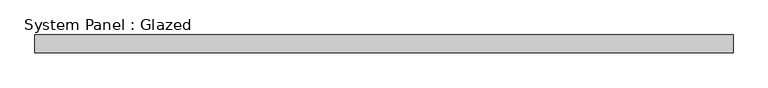
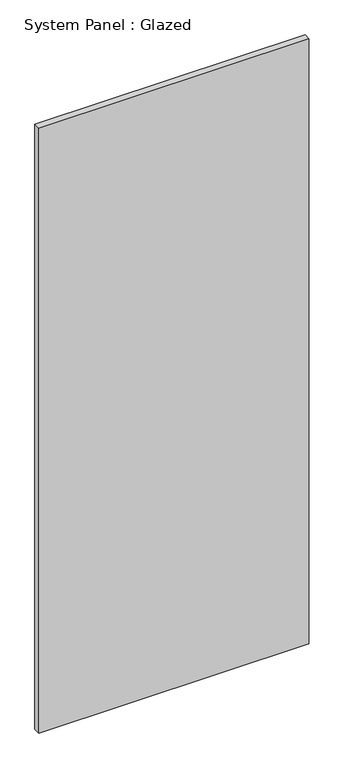
"""IFC4 building model written with IfcOpenShell, lengths in millimetres: plate geometry, System Panel : Glazed."""

from ifc_helpers import new_model, si_unit, origin, origin_with_axes, place, context, project, spatial, polyline, outline, extrude, source, transform, mapped, element, save


def system_panel_glazed_9df4f396(model_context):
    return source(origin(), model_context, "Body", "SweptSolid", [
        extrude(outline(polyline([(501.65, 19.05), (-501.65, 19.05), (-501.65, 44.45), (501.65, 44.45), (501.65, 19.05)])), origin_with_axes(), (0.0, 0.0, 1.0), 2374.9),
    ])


if __name__ == "__main__":
    model = new_model("IFC4")
    model_context = context("Model", 3, world=origin())
    ifc_project = project(units=[si_unit("LENGTHUNIT", "METRE", prefix="MILLI")], contexts=[model_context])
    site = spatial("IfcSite", under=ifc_project)
    building = spatial("IfcBuilding", under=site)
    placement = place(None, origin())
    system_panel_glazed_shape = system_panel_glazed_9df4f396(model_context)
    element("IfcPlate", 1, ObjectType="System Panel : Glazed", at=placement, inside=building, context=model_context, shape_type="MappedRepresentation", body=[
        mapped(system_panel_glazed_shape, transform((0.0, 0.0, 0.0), x_axis=(1.0, 0.0, 0.0), y_axis=(0.0, 1.0, 0.0), z_axis=(0.0, 0.0, 1.0))),
    ])
    save(model, "model.ifc")

# Revit data of these elements
# Type "System Panel : Glazed"
#   Construction Type Id = "GSP4R"
#   Analytic Construction = "1/8 in Pilkington single glazing"
#   Visual Light Transmittance = 0.9
#   Solar Heat Gain Coefficient = 0.86
#   Heat Transfer Coefficient (U) = 1.18115 BTU/(h·ft²·°F)
# Element 1 (IfcPlate, "System Panel : Glazed")
#   Materials on its faces: "Glass"
# Materials
#   "Glass": class "Glass", colour RGB 0 128 192, transparency 0.75, Description = "Soda Lime Glass", Cost = 0
